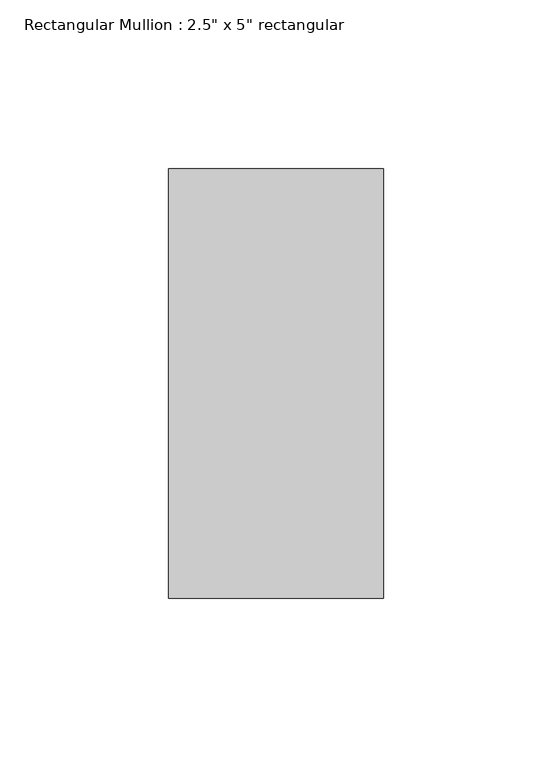
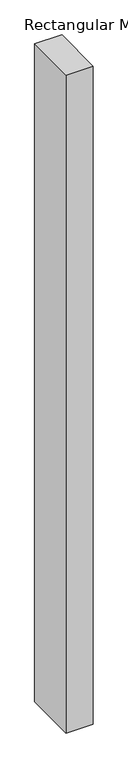
"""IFC4 building model written with IfcOpenShell, lengths in millimetres: member geometry."""

from ifc_helpers import new_model, si_unit, frame, origin, place, context, project, spatial, polyline, outline, extrude, source, transform, mapped, element, save


def member_b1f03c2a(model_context):
    return source(origin(), model_context, "Body", "SweptSolid", [
        extrude(outline(polyline([(31.75, 63.5), (31.75, -63.5), (-31.75, -63.5), (-31.75, 63.5), (31.75, 63.5)])), frame((0.0, 0.0, -1629.0255085), z_axis=(0.0, 0.0, 1.0), x_axis=(1.0, 0.0, 0.0)), (0.0, 0.0, 1.0), 1629.0255085),
    ])


if __name__ == "__main__":
    model = new_model("IFC4")
    model_context = context("Model", 3, world=origin())
    ifc_project = project(units=[si_unit("LENGTHUNIT", "METRE", prefix="MILLI")], contexts=[model_context])
    site = spatial("IfcSite", under=ifc_project)
    building = spatial("IfcBuilding", under=site)
    placement = place(None, origin())
    member_shape = member_b1f03c2a(model_context)
    element("IfcMember", 1, ObjectType="Rectangular Mullion : 2.5\" x 5\" rectangular", at=placement, inside=building, context=model_context, shape_type="MappedRepresentation", body=[
        mapped(member_shape, transform((0.0, 0.0, 0.0), x_axis=(1.0, 0.0, 0.0), y_axis=(0.0, 1.0, 0.0), z_axis=(0.0, 0.0, 1.0))),
    ])
    save(model, "model.ifc")

# Revit data of these elements
# Type "Rectangular Mullion : 2.5\" x 5\" rectangular"
#   built-in parameter 1007304 = 0.416667 (stored number, unit not read)
#   built-in parameter 1007301 = 0.104167 (stored number, unit not read)
#   built-in parameter 1007300 = 0.104167 (stored number, unit not read)
# Element 1 (IfcMember, "Rectangular Mullion : 2.5\" x 5\" rectangular")
#   Materials on its faces: "Aluminum"
# Materials
#   "Aluminum": class "Metal", colour RGB 247 247 247, transparency 0, Description = "Aluminum 6061", Cost = 0
